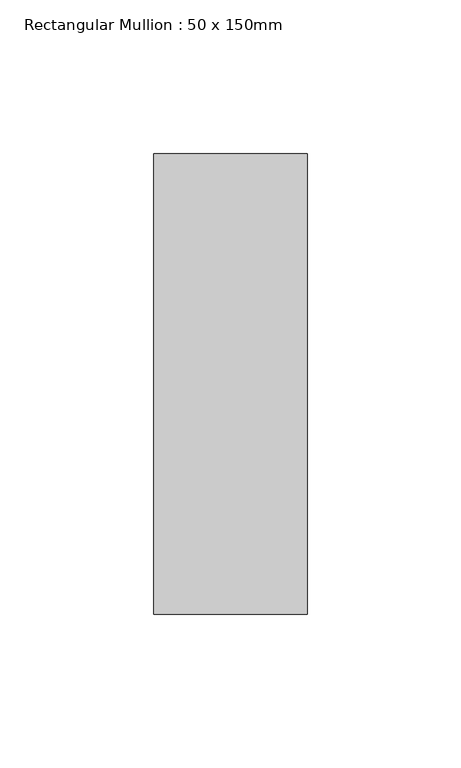
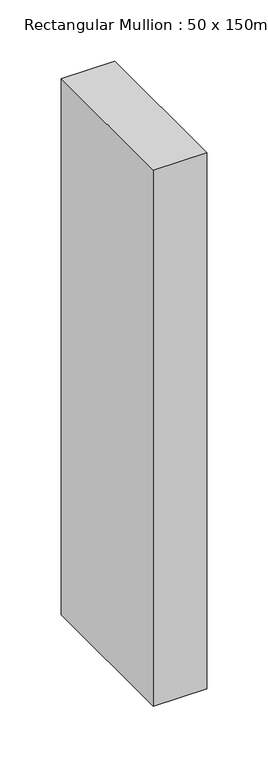
"""IFC4 building model written with IfcOpenShell, lengths in millimetres: member geometry, Rectangular Mullion : 50 x 150mm."""

from ifc_helpers import new_model, si_unit, frame, origin, place, context, project, spatial, polyline, outline, extrude, source, transform, mapped, element, save


def rectangular_mullion_50_x_150mm_15474f2d(model_context):
    return source(origin(), model_context, "Body", "SweptSolid", [
        extrude(outline(polyline([(0.0, 75.0), (0.0, -75.0), (-50.0, -75.0), (-50.0, 75.0), (0.0, 75.0)])), frame((0.0, 0.0, -533.4), z_axis=(0.0, 0.0, 1.0), x_axis=(1.0, 0.0, 0.0)), (0.0, 0.0, 1.0), 533.4),
    ])


if __name__ == "__main__":
    model = new_model("IFC4")
    model_context = context("Model", 3, world=origin())
    ifc_project = project(units=[si_unit("LENGTHUNIT", "METRE", prefix="MILLI")], contexts=[model_context])
    site = spatial("IfcSite", under=ifc_project)
    building = spatial("IfcBuilding", under=site)
    placement = place(None, origin())
    rectangular_mullion_50_x_150mm_shape = rectangular_mullion_50_x_150mm_15474f2d(model_context)
    element("IfcMember", 1, ObjectType="Rectangular Mullion : 50 x 150mm", at=placement, inside=building, context=model_context, shape_type="MappedRepresentation", body=[
        mapped(rectangular_mullion_50_x_150mm_shape, transform((0.0, 0.0, 0.0), x_axis=(1.0, 0.0, 0.0), y_axis=(0.0, 1.0, 0.0), z_axis=(0.0, 0.0, 1.0))),
    ])
    save(model, "model.ifc")

# Revit data of these elements
# Type "Rectangular Mullion : 50 x 150mm"
#   built-in parameter 1007304 = 0.492126 (stored number, unit not read)
#   built-in parameter 1007301 = 0.082021 (stored number, unit not read)
#   built-in parameter 1007300 = 0.082021 (stored number, unit not read)
# Element 1 (IfcMember, "Rectangular Mullion : 50 x 150mm")
#   Materials on its faces: "Aluminium"
# Materials
#   "Aluminium": class "Metal", colour RGB 247 247 247, transparency 0, Description = "Aluminium 6061", Cost = 0
